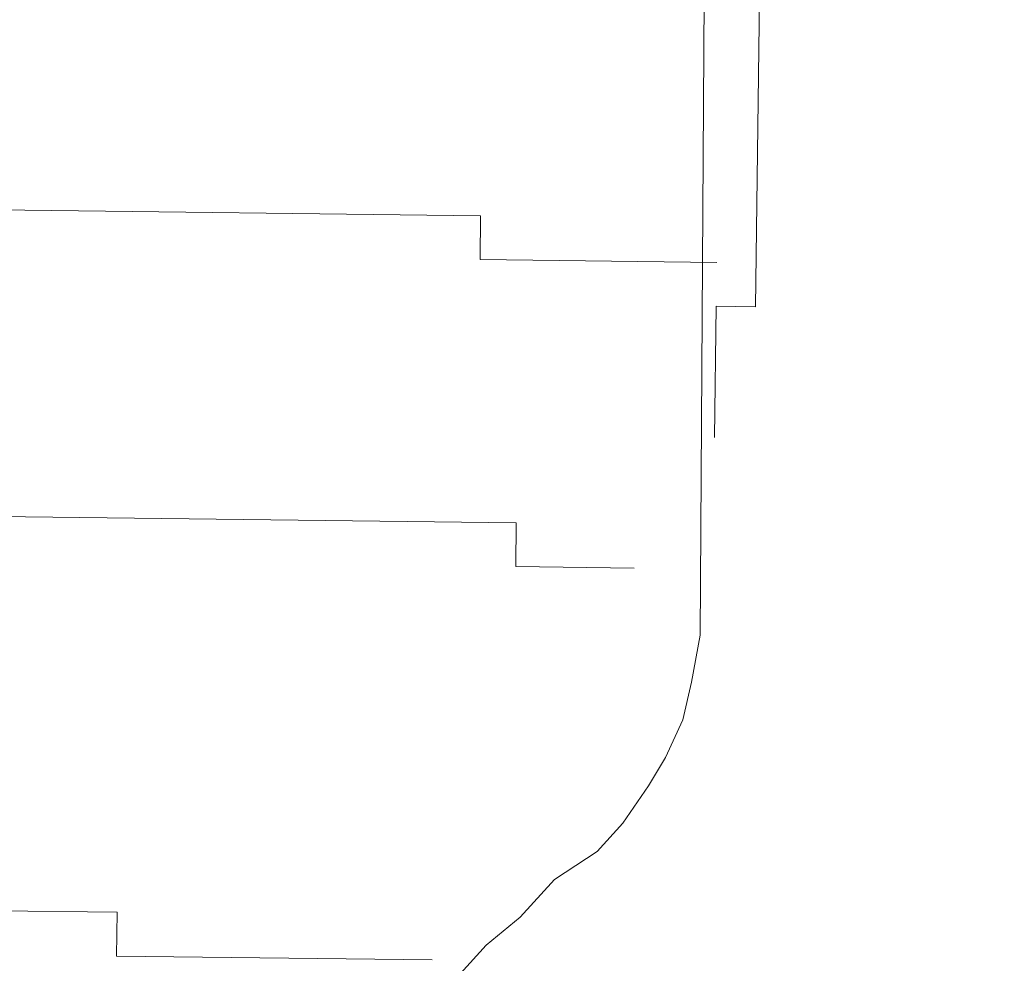
# Model space of a CAD drawing. Units: inches. Extents: x -466983 to 1020, y 324 to 318697.
# Tile 63 of 97: x 640.735 to 643.839, y 942.694 to 945.669. Entities that reach past the tile are written whole.
import ezdxf

# ---------------------------------------------------------------- set-up
doc = ezdxf.new("R2010")
doc.units = ezdxf.units.IN
doc.header["$MEASUREMENT"] = 0
doc.layers.add('A-FLOR-PATT', color=252, linetype='Continuous', lineweight=13)
doc.layers.add('A-FURN', color=8, linetype='Continuous', lineweight=18)

# ---------------------------------------------------------------- blocks, each defined once
blk = doc.blocks.new('L Shaped Sofa')
at = {"ltscale": 2}
for p, q in [((2421.6339, 743.6354), (2421.7812, 743.7974)), ((2421.9449, 743.7202), (2423.7596, 743.698)), ((2423.7596, 743.698), (2423.7566, 743.4461)), ((2421.4377, 743.4737), (2421.6339, 743.6354)), ((2421.2412, 743.2577), (2421.4377, 743.4737)), ((2423.7566, 743.4461), (2430.7885, 743.3602)), ((2420.9962, 743.0962), (2421.2412, 743.2577)), ((2420.8488, 742.9343), (2420.9962, 743.0962)), ((2420.7011, 742.7181), (2420.8488, 742.9343)), ((2420.6025, 742.5559), (2420.7011, 742.7181)), ((2420.5036, 742.3395), (2420.6025, 742.5559)), ((2420.4535, 742.1229), (2420.5036, 742.3395)), ((2420.403, 741.852), (2420.4535, 742.1229)), ((2420.3785, 737.84), (2420.403, 741.852)), ((2420.7831, 741.4668), (2421.4636, 741.4585)), ((2421.4636, 741.4585), (2421.4605, 741.2066)), ((2421.4605, 741.2066), (2432.3486, 741.0736)), ((2420.3109, 739.9609), (2420.3202, 740.7166)), ((2420.0564, 737.6965), (2420.0841, 739.9637)), ((2420.0841, 739.9637), (2420.3109, 739.9609)), ((2420.3078, 739.709), (2421.6689, 739.6924)), ((2421.6689, 739.6924), (2421.6658, 739.4404)), ((2421.6658, 739.4404), (2428.4709, 739.3573))]:
    blk.add_line(p, q, dxfattribs=at)

msp = doc.modelspace()

# ---------------------------------------------------------------- hatches: boundary and pattern name
at = {"layer": 'A-FLOR-PATT', "transparency": 33554572}
h = msp.add_hatch(dxfattribs=at)
h.set_pattern_fill('ANSI37', color=256, scale=30)
h.set_pattern_definition([(45, (-1212.4137, -290.035), (-2.6516504, 2.6516504), []), (135, (-1212.4137, -290.035), (-2.6516504, -2.6516504), [])])
h.paths.add_polyline_path([(901.8057, 1075.9377), (900.6144, 1075.9377), (900.6144, 1065.3856), (899.391, 1065.3856), (898.0911, 1065.3856), (892.8356, 1058.7098, -0.258377), (892.1875, 1058.3509), (879.9848, 1058.3509, -0.20177), (879.4382, 1058.5808), (874.0812, 1065.3856), (872.7813, 1065.3856), (871.5579, 1065.3856), (871.5579, 1075.9377), (813.8057, 1075.9377), (813.8057, 1044.7922), (832.3947, 1044.7922, -0.394795), (848.6602, 1028.5356), (848.6602, 1009.9377), (901.8057, 1009.9377), (901.8057, 1015.9377), (901.3057, 1015.9377), (871.3057, 1015.9377), (871.3057, 1017.2502), (871.3344, 1017.2502, -0.401453), (901.3057, 1045.9377), (901.8057, 1045.9377)])
edge = h.paths.add_edge_path(flags=16)
edge.add_line((847.7731, 1068.9486), (847.7731, 1073.7088))
edge.add_arc((849.2269, 1073.7088), 1.4538, 90, 180, ccw=False)
edge.add_line((849.2269, 1075.1627), (864.4921, 1075.1627))
edge.add_arc((864.4921, 1073.7088), 1.4538, 0, 90, ccw=False)
edge.add_line((865.9459, 1073.7088), (865.9459, 1069.0035))
edge.add_arc((832.6447, 1068.9761), 33.3012, -20.61234, 0.04725, ccw=False)
edge.add_ellipse((856.8595, 1058.48), major_axis=(0, 10.2131), ratio=0.6859192, start_angle=100.00884, end_angle=259.99116, ccw=False)
edge.add_arc((881.0742, 1068.9761), 33.3012, 180.04725, 200.61234, ccw=False)
h.paths.add_polyline_path([(853.1456, 1066.4815), (853.1456, 1066.4534), (853.1463, 1066.4534, 0.433107), (852.9166, 1066.6849), (852.9166, 1066.4534), (853.1456, 1066.4534), (853.1456, 1066.4815), (853.088, 1066.6122, 0.697939), (852.6995, 1066.4534), (852.7003, 1066.4534), (852.7003, 1066.4815), (852.9166, 1067.0012), (852.9166, 1066.6849, -0.396254)], flags=0)
h.paths.add_polyline_path([(861.0187, 1066.4815), (861.0187, 1066.4534), (861.0194, 1066.4534, 0.416404), (860.8024, 1066.6849), (860.8024, 1066.4534), (861.0187, 1066.4534), (861.0187, 1066.4815), (860.9672, 1066.6053, 0.713344), (860.5726, 1066.4534), (860.5734, 1066.4534), (860.5734, 1066.4815), (860.8024, 1067.0012), (860.8024, 1066.6849, -0.379973)], flags=0)
edge = h.paths.add_edge_path(flags=0)
edge.add_spline(control_points=[(861.1298, 1065.7855), (861.4661, 1065.2478), (861.6134, 1065.0161), (861.9833, 1064.3736), (862.1924, 1063.9443), (862.5614, 1063.0391), (862.7212, 1062.5633), (862.9865, 1061.5781), (863.092, 1061.0689), (863.2452, 1060.031), (863.293, 1059.5025), (863.3295, 1058.4409), (863.3181, 1057.9078), (863.2366, 1056.8518), (863.1664, 1056.3289), (862.9695, 1055.308), (862.8427, 1054.8099), (862.5365, 1053.8522), (862.3571, 1053.3927), (861.9514, 1052.5249), (861.7251, 1052.1166), (861.233, 1051.3622), (860.9672, 1051.0162), (860.4048, 1050.3949), (860.1082, 1050.1197), (859.4937, 1049.6461), (859.1758, 1049.4476), (858.5276, 1049.1299), (858.1973, 1049.0107), (857.5315, 1048.8518), (857.1959, 1048.8121), (856.5249, 1048.812), (856.1894, 1048.8515), (855.5236, 1049.0101), (855.1933, 1049.1291), (854.545, 1049.4465), (854.2271, 1049.6449), (853.6124, 1050.1183), (853.3158, 1050.3933), (852.7533, 1051.0143), (852.4874, 1051.3602), (851.9952, 1052.1144), (851.7688, 1052.5225), (851.3629, 1053.3902), (851.1834, 1053.8496), (850.877, 1054.8071), (850.7501, 1055.3051), (850.553, 1056.326), (850.4827, 1056.8488), (850.401, 1057.9048), (850.3895, 1058.4379), (850.4257, 1059.4995), (850.4734, 1060.0281), (850.6265, 1061.066), (850.7318, 1061.5753), (850.9969, 1062.5605), (851.1567, 1063.0365), (851.5254, 1063.9418), (851.7345, 1064.3712), (852.1056, 1065.0164), (852.2544, 1065.2503), (852.6082, 1065.7335)], knot_values=[3.915332, 3.915332, 3.915332, 3.915332, 4.013468, 4.013468, 4.175532, 4.175532, 4.337596, 4.337596, 4.49966, 4.49966, 4.661724, 4.661724, 4.823788, 4.823788, 4.985852, 4.985852, 5.147916, 5.147916, 5.30998, 5.30998, 5.472044, 5.472044, 5.634109, 5.634109, 5.796173, 5.796173, 5.958237, 5.958237, 6.120301, 6.120301, 6.282365, 6.282365, 6.444429, 6.444429, 6.606493, 6.606493, 6.768557, 6.768557, 6.930621, 6.930621, 7.092685, 7.092685, 7.254749, 7.254749, 7.416813, 7.416813, 7.578878, 7.578878, 7.740942, 7.740942, 7.903006, 7.903006, 8.06507, 8.06507, 8.227134, 8.227134, 8.389198, 8.389198, 8.551262, 8.551262, 8.65037, 8.65037, 8.65037, 8.65037], degree=3, periodic=0)
edge.add_line((852.6421, 1065.7855), (861.1298, 1065.7855))
edge = h.paths.add_edge_path(flags=0)
edge.add_ellipse((856.8496, 1057.7432), major_axis=(0, 7.7921), ratio=0.687861, start_angle=0, end_angle=360)
h.paths.add_polyline_path([(848.8634, 1069.3891), (848.8634, 1073.9605, -0.414214), (849.9538, 1075.0508), (863.7652, 1075.0508, -0.414214), (864.8555, 1073.9605), (864.8555, 1069.3891, -0.388936), (864.5237, 1069.027, -0.043561), (849.1953, 1069.027, -0.388936)], flags=0)
h.paths.add_polyline_path([(853.1006, 1068.1122, -1), (852.6775, 1068.1122, -1)], flags=0)
edge = h.paths.add_edge_path(flags=0)
edge.add_ellipse((856.8595, 1057.3378), major_axis=(0, 2.207), ratio=0.657164, start_angle=0, end_angle=360)
h.paths.add_polyline_path([(861.0415, 1068.1122, -1), (860.6184, 1068.1122, -1)], flags=0)
edge = h.paths.add_edge_path()
edge.add_line((573.9537, 1057.3412), (573.9537, 1075.9377))
edge.add_line((573.9537, 1075.9377), (558.7308, 1075.9377))
edge.add_line((558.7308, 1075.9377), (558.7308, 1065.3856))
edge.add_line((558.7308, 1065.3856), (557.5074, 1065.3856))
edge.add_line((557.5074, 1065.3856), (556.2075, 1065.3856))
edge.add_line((556.2075, 1065.3856), (550.952, 1058.7098))
edge.add_arc((550.3039, 1059.1155), 0.7646, 270, 327.9483, ccw=False)
edge.add_line((550.3039, 1058.3509), (538.1012, 1058.3509))
edge.add_arc((538.1012, 1059.1155), 0.7646, 224.3704, 270, ccw=False)
edge.add_line((537.5546, 1058.5808), (532.1976, 1065.3856))
edge.add_line((532.1976, 1065.3856), (530.8977, 1065.3856))
edge.add_line((530.8977, 1065.3856), (529.6743, 1065.3856))
edge.add_line((529.6743, 1065.3856), (529.6743, 1075.9377))
edge.add_line((529.6743, 1075.9377), (520.8057, 1075.9377))
edge.add_line((520.8057, 1075.9377), (520.8057, 1045.9377))
edge.add_line((520.8057, 1045.9377), (521.3057, 1045.9377))
edge.add_arc((521.3057, 1015.9377), 30, 2.50749, 90, ccw=False)
edge.add_line((551.277, 1017.2502), (551.3057, 1017.2502))
edge.add_line((551.3057, 1017.2502), (551.3057, 1015.9377))
edge.add_line((551.3057, 1015.9377), (520.8057, 1015.9377))
edge.add_line((520.8057, 1015.9377), (520.8057, 1009.9377))
edge.add_line((520.8057, 1009.9377), (559.1913, 1010.4022))
edge.add_arc((559.1913, 1011.856), 1.4538, 180, 270, ccw=False)
edge.add_line((557.7375, 1011.856), (557.7375, 1016.5613))
edge.add_arc((591.0386, 1016.5888), 33.3012, 159.38766, 180.04725, ccw=False)
edge.add_ellipse((566.8239, 1027.0848), major_axis=(0, 10.2131), ratio=0.6859192, start_angle=280.00884, end_angle=439.99116, ccw=False)
edge.add_arc((542.6091, 1016.5888), 33.3012, 0.04725, 20.61234, ccw=False)
edge.add_line((575.9103, 1016.6162), (575.9103, 1011.856))
edge.add_arc((574.4565, 1011.856), 1.4538, -90, 0, ccw=False)
edge.add_line((574.4565, 1010.4022), (608.8057, 1009.9377))
edge.add_line((608.8057, 1009.9377), (608.8057, 1041.0857))
edge.add_line((608.8057, 1041.0857), (590.2179, 1041.0857))
edge.add_arc((590.775, 1057.9074), 16.8309, 181.92775, 268.10321, ccw=False)
edge = h.paths.add_edge_path()
edge.add_ellipse((494.2443, 583.6204), major_axis=(0, 10.2131), ratio=0.6859192, start_angle=280.00884, end_angle=439.99116, ccw=False)
edge.add_arc((470.0296, 573.1243), 33.3012, 0.04725, 20.61234, ccw=False)
edge.add_line((503.3307, 573.1518), (503.3307, 568.3916))
edge.add_arc((501.8769, 568.3916), 1.4538, -90, 0, ccw=False)
edge.add_line((501.8769, 566.9377), (539.8057, 566.9377))
edge.add_line((539.8057, 566.9377), (539.8057, 572.9377))
edge.add_line((539.8057, 572.9377), (539.3057, 572.9377))
edge.add_line((539.3057, 572.9377), (509.3057, 572.9377))
edge.add_line((509.3057, 572.9377), (509.3057, 574.2502))
edge.add_line((509.3057, 574.2502), (509.3344, 574.2502))
edge.add_arc((539.3057, 572.9377), 30, 90, 177.49251, ccw=False)
edge.add_line((539.3057, 602.9377), (539.8057, 602.9377))
edge.add_line((539.8057, 602.9377), (539.8057, 626.9377))
edge.add_line((539.8057, 626.9377), (531.7718, 626.9377))
edge.add_line((531.7718, 626.9377), (531.7718, 616.3856))
edge.add_line((531.7718, 616.3856), (530.5484, 616.3856))
edge.add_line((530.5484, 616.3856), (529.2485, 616.3856))
edge.add_line((529.2485, 616.3856), (523.7105, 609.3509))
edge.add_line((523.7105, 609.3509), (510.7766, 609.3509))
edge.add_line((510.7766, 609.3509), (505.2386, 616.3856))
edge.add_line((505.2386, 616.3856), (503.9387, 616.3856))
edge.add_line((503.9387, 616.3856), (502.7153, 616.3856))
edge.add_line((502.7153, 616.3856), (502.7153, 626.9377))
edge.add_line((502.7153, 626.9377), (481.6983, 626.9377))
edge.add_line((481.6983, 626.9377), (481.6983, 610.995))
edge.add_arc((467.2703, 611.4728), 14.4359, 271.92775, 358.10321, ccw=False)
edge.add_line((467.7559, 597.0451), (451.8057, 597.0451))
edge.add_line((451.8057, 597.0451), (451.8057, 584.4035))
edge.add_line((451.8057, 584.4035), (451.8057, 566.9377))
edge.add_line((451.8057, 566.9377), (486.6117, 566.9377))
edge.add_arc((486.6117, 568.3916), 1.4538, 180, 270, ccw=False)
edge.add_line((485.1579, 568.3916), (485.1579, 573.0969))
edge.add_arc((518.4591, 573.1243), 33.3012, 159.38766, 180.04725, ccw=False)
h.paths.add_polyline_path([(836.2609, 1020.7328), (879.8898, 1020.7328), (879.8898, 1039.3902), (836.2609, 1039.3902)], flags=25)
h.paths.add_polyline_path([(549.9851, 1036.7492), (593.614, 1036.7492), (593.614, 1055.4065), (549.9851, 1055.4065)], flags=24)
h.paths.add_polyline_path([(475.123, 595.5959), (518.752, 595.5959), (518.752, 614.2532), (475.123, 614.2532)], flags=24)
h = msp.add_hatch(dxfattribs=at)
h.set_pattern_fill('ANSI37', color=256, scale=20)
h.set_pattern_definition([(45, (-1212.4137, -290.035), (-1.767767, 1.767767), []), (135, (-1212.4137, -290.035), (-1.767767, -1.767767), [])])
h.paths.add_polyline_path([(809.8057, 870.9377), (809.8057, 888.1519), (806.9985, 888.1519), (802.6624, 888.1519), (789.3832, 888.1519), (786.2846, 888.1519, -0.414214), (785.4991, 888.9374), (785.4991, 900.1959), (785.4991, 908.4696, -0.414214), (786.8082, 909.7787, -0.414214), (785.4991, 911.0878), (785.4991, 929.1015, -0.414214), (786.8082, 930.4106, -0.414214), (785.4991, 931.7197), (785.4991, 931.9039, -0.414214), (784.19, 930.5948), (766.7223, 930.5948, -0.412359), (765.4132, 931.8956, -0.413741), (764.1145, 930.5782), (744.5781, 930.422, -0.416556), (743.7864, 931.2075), (743.7864, 933.5153), (742.2154, 933.5153), (742.2154, 952.024, -0.001344), (743.7864, 952.1998), (743.7864, 953.9377), (678.5915, 953.9377), (678.5915, 951.1305), (678.5915, 946.7945), (678.5915, 933.5153), (678.5915, 930.4166, -0.414214), (677.806, 929.6312), (666.5475, 929.6312), (658.2738, 929.6312, -0.414214), (656.9647, 930.9403, -0.414214), (655.6556, 929.6312), (637.6419, 929.6312, -0.414214), (636.3328, 930.9403, -0.414214), (635.0237, 929.6312), (634.8395, 929.6312, -0.414214), (636.1486, 928.322), (636.1486, 910.8544, -0.412359), (634.8478, 909.5452, -0.413741), (636.1653, 908.2466), (636.3214, 888.7102, -0.416556), (635.5359, 887.9184), (633.2281, 887.9184), (633.2281, 886.3475), (614.7194, 886.3475, -0.001344), (614.5436, 887.9184), (612.8057, 887.9184), (612.8057, 834.9377), (612.8057, 752.9377), (612.8057, 748.9377), (612.8057, 697.9377), (654.8057, 697.9377), (654.8057, 701.9377), (715.8057, 701.9377), (715.8057, 737.4353), (774.2918, 737.4353), (774.2918, 795.9377), (809.8057, 795.9377)])
h.paths.add_polyline_path([(679.2761, 849.5757, 0.102523), (682.1475, 849.2608, -0.080461), (694.5428, 849.7725, -0.283899), (694.4822, 849.0082, 0.136605), (694.4068, 848.8103, -0.030441), (694.5428, 846.8929), (694.5428, 842.6198), (694.5428, 838.3466, -0.028219), (694.4246, 836.5684), (694.425, 836.5684, 0.196187), (694.4456, 836.2708, -0.302897), (694.5428, 835.467, -0.080461), (682.1475, 835.9787, 0.102523), (679.2761, 835.6638, -0.58611), (678.6457, 836.0169), (678.6457, 849.2227, -0.58611)], flags=16)
h.paths.add_polyline_path([(679.5173, 848.6515, 0.699597), (679.476, 848.6342, 1.20716), (679.1935, 848.7422, 0.010621)], flags=0)
h.paths.add_polyline_path([(679.4923, 836.5608, -0.013798), (679.9178, 836.6594, -0.071703), (682.8533, 837.1434, -0.165743), (682.1665, 839.1006), (682.1665, 842.6094), (682.1665, 846.0603, -0.240616), (683.4733, 848.6767, -0.068263), (693.9295, 849.0082), (693.7875, 848.7083), (693.7875, 849.0228, 0.067332), (683.4733, 848.6767, 0.240616), (682.1665, 846.0603), (682.1665, 842.6094), (682.1665, 839.1006, 0.23459), (683.461, 836.5513, 0.068093), (693.7875, 836.1955), (693.7875, 836.5104), (693.9296, 836.2102, -0.077215), (682.2421, 836.7815, 0.086627), (679.5283, 836.5701, -0.628402), (679.5029, 836.5735), (679.5029, 836.6071, 0.910458)], flags=0)
h.paths.add_polyline_path([(679.476, 848.6364), (679.2069, 848.647), (679.2069, 836.5718, 0.913566), (679.3645, 836.5861), (679.476, 836.5824)], flags=0)
h.paths.add_polyline_path([(679.2761, 829.8604, 0.102523), (682.1475, 829.5455, -0.080461), (694.5428, 830.0572, -0.283899), (694.4822, 829.2929, 0.136605), (694.4068, 829.095, -0.030441), (694.5428, 827.1776), (694.5428, 822.9045), (694.5428, 818.6314, -0.028219), (694.4246, 816.8531), (694.425, 816.8532, 0.196187), (694.4456, 816.5555, -0.302897), (694.5428, 815.7517, -0.080461), (682.1475, 816.2635, 0.102523), (679.2761, 815.9485, -0.58611), (678.6457, 816.3016), (678.6457, 829.5074, -0.58611)], flags=16)
h.paths.add_polyline_path([(679.5173, 828.9362, 0.699597), (679.476, 828.9189, 1.20716), (679.1935, 829.0269, 0.010621)], flags=0)
h.paths.add_polyline_path([(679.4923, 816.8456, -0.013798), (679.9178, 816.9441, -0.071703), (682.8533, 817.4281, -0.165743), (682.1665, 819.3853), (682.1665, 822.8941), (682.1665, 826.345, -0.240616), (683.4733, 828.9614, -0.068263), (693.9295, 829.2929), (693.7875, 828.9931), (693.7875, 829.3076, 0.067332), (683.4733, 828.9614, 0.240616), (682.1665, 826.345), (682.1665, 822.8941), (682.1665, 819.3853, 0.23459), (683.461, 816.836, 0.068093), (693.7875, 816.4802), (693.7875, 816.7952), (693.9296, 816.4949, -0.077215), (682.2421, 817.0662, 0.086627), (679.5283, 816.8549, -0.628402), (679.5029, 816.8582), (679.5029, 816.8918, 0.910458)], flags=0)
h.paths.add_polyline_path([(679.476, 828.9211), (679.2069, 828.9317), (679.2069, 816.8565, 0.913566), (679.3645, 816.8708), (679.476, 816.8671)], flags=0)
h.paths.add_polyline_path([(679.2761, 810.1451, 0.102523), (682.1475, 809.8302, -0.080461), (694.5428, 810.342, -0.3023), (694.4466, 809.5394, 0.10023), (694.4058, 809.3878, -0.03057), (694.5428, 807.4623), (694.5428, 803.1892), (694.5428, 798.9161, -0.03057), (694.4058, 796.9906, 0.10023), (694.4466, 796.839, -0.3023), (694.5428, 796.0365, -0.080461), (682.1475, 796.5482, 0.102523), (679.2761, 796.2333, -0.58611), (678.6457, 796.5863), (678.6457, 809.7921, -0.58611)], flags=16)
h.paths.add_polyline_path([(679.5173, 809.2417, 0.699597), (679.476, 809.2244, 1.20716), (679.1935, 809.3324, 0.010621)], flags=0)
h.paths.add_polyline_path([(679.4923, 797.151, -0.013798), (679.9178, 797.2496, -0.071703), (682.8533, 797.7336, -0.165743), (682.1665, 799.6908), (682.1665, 803.1996), (682.1665, 806.6505, -0.239349), (683.461, 809.2577, -0.072465), (694.4468, 809.5405, 0.197932), (694.425, 809.2405), (693.7875, 809.2985), (693.7875, 809.6135, 0.068093), (683.461, 809.2577, 0.239349), (682.1665, 806.6505), (682.1665, 803.1996), (682.1665, 799.6908, 0.235854), (683.4733, 797.1323, 0.067332), (693.7875, 796.7861), (693.7875, 797.1006), (694.425, 797.1586, 0.197932), (694.4468, 796.8586, -0.080419), (682.1557, 797.3795, 0.083867), (679.5283, 797.1603, -0.628402), (679.5029, 797.1637), (679.5029, 797.1973, 0.910458)], flags=0)
h.paths.add_polyline_path([(679.2069, 809.2372), (679.2069, 797.162, 0.913566), (679.3645, 797.1763), (679.476, 797.1726), (679.476, 809.2266)], flags=0)
h.paths.add_polyline_path([(695.3643, 853.2989), (728.2231, 853.2989), (728.2231, 771.1519), (695.3643, 771.1519)], flags=16)
h.paths.add_polyline_path([(696.0215, 852.6417), (727.5659, 852.6417), (727.5659, 771.809), (696.0215, 771.809)], flags=0)
h.paths.add_polyline_path([(679.2761, 788.7869, 0.102523), (682.1475, 788.472, -0.080461), (694.5428, 788.9837, -0.3023), (694.4466, 788.1812, 0.10023), (694.4058, 788.0296, -0.03057), (694.5428, 786.1041), (694.5428, 781.831), (694.5428, 777.5578, -0.03057), (694.4058, 775.6323, 0.10023), (694.4466, 775.4808, -0.3023), (694.5428, 774.6782, -0.080461), (682.1475, 775.19, 0.102523), (679.2761, 774.875, -0.58611), (678.6457, 775.2281), (678.6457, 788.4339, -0.58611)], flags=16)
h.paths.add_polyline_path([(679.5173, 787.8834, 0.699597), (679.476, 787.8662, 1.20716), (679.1935, 787.9742, 0.010621)], flags=0)
h.paths.add_polyline_path([(679.4923, 775.7928, -0.013798), (679.9178, 775.8914, -0.071703), (682.8533, 776.3753, -0.165743), (682.1665, 778.3325), (682.1665, 781.8414), (682.1665, 785.2922, -0.239349), (683.461, 787.8995, -0.072465), (694.4468, 788.1823, 0.197932), (694.425, 787.8823), (693.7875, 787.9403), (693.7875, 788.2553, 0.068093), (683.461, 787.8995, 0.239349), (682.1665, 785.2922), (682.1665, 781.8414), (682.1665, 778.3325, 0.235854), (683.4733, 775.7741, 0.067332), (693.7875, 775.4279), (693.7875, 775.7424), (694.425, 775.8004, 0.197932), (694.4468, 775.5004, -0.080419), (682.1557, 776.0212, 0.083867), (679.5283, 775.8021, -0.628402), (679.5029, 775.8054), (679.5029, 775.8391, 0.910458)], flags=0)
h.paths.add_polyline_path([(679.2069, 787.8789), (679.2069, 775.8038, 0.913566), (679.3645, 775.818), (679.476, 775.8144), (679.476, 787.8684)], flags=0)
h.paths.add_polyline_path([(704.641, 854.1204, -0.080461), (705.1527, 866.5157, 0.102523), (704.8378, 869.3871, -0.58611), (705.1908, 870.0174), (718.3966, 870.0174, -0.58611), (718.7496, 869.3871, 0.102523), (718.4347, 866.5157, -0.080461), (718.9465, 854.1204, -0.3023), (718.1439, 854.2166, 0.10023), (717.9924, 854.2574, -0.03057), (716.0668, 854.1204), (711.7937, 854.1204), (707.5206, 854.1204, -0.03057), (705.5951, 854.2574, 0.10023), (705.4435, 854.2166, -0.3023)], flags=16)
h.paths.add_polyline_path([(717.8462, 869.1459, 0.699597), (717.8289, 869.1872, 1.20716), (717.9369, 869.4697, 0.010621)], flags=0)
h.paths.add_polyline_path([(705.4631, 854.2164, -0.080419), (705.984, 866.5074, 0.083867), (705.7648, 869.1349, -0.628402), (705.7682, 869.1603), (705.8018, 869.1603, 0.910458), (705.7555, 869.1709, -0.013798), (705.8541, 868.7454, -0.071703), (706.3381, 865.8099, -0.165743), (708.2953, 866.4967), (711.8041, 866.4967), (715.255, 866.4967, -0.239349), (717.8622, 865.2022, -0.072465), (718.145, 854.2164, 0.197932), (717.845, 854.2382), (717.903, 854.8757), (718.218, 854.8757, 0.068093), (717.8622, 865.2022, 0.239349), (715.255, 866.4967), (711.8041, 866.4967), (708.2953, 866.4967, 0.235854), (705.7368, 865.1898, 0.067332), (705.3906, 854.8757), (705.7051, 854.8757), (705.7631, 854.2382, 0.197932)], flags=16)
h.paths.add_polyline_path([(705.7665, 869.4563, 0.913566), (705.7808, 869.2987), (705.7771, 869.1872), (717.8311, 869.1872), (717.8417, 869.4563)], flags=0)
h.paths.add_polyline_path([(729.0446, 842.6198), (729.0446, 846.8929, -0.03057), (729.1817, 848.8184, 0.10023), (729.1408, 848.9699, -0.3023), (729.0446, 849.7725, -0.080461), (741.4399, 849.2608, 0.102523), (744.3113, 849.5757, -0.58611), (744.9417, 849.2227), (744.9417, 836.0169, -0.58611), (744.3113, 835.6638, 0.102523), (741.4399, 835.9787, -0.080461), (729.0446, 835.467, -0.3023), (729.1408, 836.2696, 0.10023), (729.1817, 836.4211, -0.03057), (729.0446, 838.3466)], flags=16)
h.paths.add_polyline_path([(744.1115, 836.5846, 1.20716), (744.3939, 836.4766, 0.010621), (744.0701, 836.5673, 0.699597)], flags=0)
h.paths.add_polyline_path([(729.1407, 836.2684, 0.197932), (729.1624, 836.5684), (729.7999, 836.5104), (729.7999, 836.1955, 0.068093), (740.1264, 836.5513, 0.239349), (741.4209, 839.1585), (741.4209, 842.6094), (741.4209, 846.1182, 0.235854), (740.1141, 848.6767, 0.067332), (729.7999, 849.0228), (729.7999, 848.7083), (729.1624, 848.6503, 0.197932), (729.1407, 848.9504, -0.080419), (741.4317, 848.4295, 0.083867), (744.0591, 848.6486, -0.628402), (744.0845, 848.6453), (744.0845, 848.6117, 0.910458), (744.0951, 848.6579, -0.013798), (743.6696, 848.5594, -0.071703), (740.7341, 848.0754, -0.165743), (741.4209, 846.1182), (741.4209, 842.6094), (741.4209, 839.1585, -0.239349), (740.1264, 836.5513, -0.072465)], flags=0)
h.paths.add_polyline_path([(729.0446, 830.0572, -0.080461), (741.4399, 829.5455, 0.102523), (744.3113, 829.8604, -0.58611), (744.9417, 829.5074), (744.9417, 816.3016, -0.58611), (744.3113, 815.9485, 0.102523), (741.4399, 816.2635, -0.080461), (729.0446, 815.7517, -0.3023), (729.1408, 816.5543, 0.10023), (729.1817, 816.7058, -0.03057), (729.0446, 818.6314), (729.0446, 822.9045), (729.0446, 827.1776, -0.03057), (729.1817, 829.1031, 0.10023), (729.1408, 829.2547, -0.3023)], flags=16)
h.paths.add_polyline_path([(744.1115, 816.8693, 1.20716), (744.3939, 816.7613, 0.010621), (744.0701, 816.852, 0.699597)], flags=0)
h.paths.add_polyline_path([(729.1407, 829.2351, -0.080419), (741.4317, 828.7142, 0.083867), (744.0591, 828.9334, -0.628402), (744.0845, 828.93), (744.0845, 828.8964, 0.910458), (744.0951, 828.9427, -0.013798), (743.6696, 828.8441, -0.071703), (740.7341, 828.3601, -0.165743), (741.4209, 826.4029), (741.4209, 822.8941), (741.4209, 819.4432, -0.239349), (740.1264, 816.836, -0.072465), (729.1407, 816.5531, 0.197932), (729.1624, 816.8532), (729.7999, 816.7952), (729.7999, 816.4802, 0.068093), (740.1264, 816.836, 0.239349), (741.4209, 819.4432), (741.4209, 822.8941), (741.4209, 826.4029, 0.235854), (740.1141, 828.9614, 0.067332), (729.7999, 829.3076), (729.7999, 828.9931), (729.1624, 828.9351, 0.197932)], flags=16)
h.paths.add_polyline_path([(729.0446, 810.342, -0.080461), (741.4399, 809.8302, 0.102523), (744.3113, 810.1451, -0.58611), (744.9417, 809.7921), (744.9417, 796.5863, -0.58611), (744.3113, 796.2333, 0.102523), (741.4399, 796.5482, -0.080461), (729.0446, 796.0365, -0.283899), (729.1052, 796.8007, 0.136605), (729.1806, 796.9987, -0.030441), (729.0446, 798.9161), (729.0446, 803.1892), (729.0446, 807.4623, -0.028219), (729.1628, 809.2406), (729.1624, 809.2405, 0.196187), (729.1418, 809.5382, -0.302897)], flags=16)
h.paths.add_polyline_path([(744.1115, 797.1748, 1.20716), (744.3939, 797.0668, 0.010621), (744.0701, 797.1575, 0.699597)], flags=0)
h.paths.add_polyline_path([(741.3453, 809.0275, 0.086627), (744.0591, 809.2388, -0.628402), (744.0845, 809.2355), (744.0845, 809.2019, 0.910458), (744.0951, 809.2481, -0.013798), (743.6696, 809.1496, -0.071703), (740.7341, 808.6656, -0.165743), (741.4209, 806.7084), (741.4209, 803.1996), (741.4209, 799.7487, -0.240616), (740.1141, 797.1323, -0.068263), (729.658, 796.8008), (729.7999, 797.1006), (729.7999, 796.7861, 0.067332), (740.1141, 797.1323, 0.240616), (741.4209, 799.7487), (741.4209, 803.1996), (741.4209, 806.7084, 0.23459), (740.1264, 809.2577, 0.068093), (729.7999, 809.6135), (729.7999, 809.2985), (729.6578, 809.5988, -0.077215)], flags=0)
h.paths.add_polyline_path([(704.641, 770.3304, -0.283899), (705.4053, 770.2697, 0.136605), (705.6032, 770.1944, -0.030441), (707.5206, 770.3304), (711.7937, 770.3304), (716.0668, 770.3304, -0.028219), (717.8451, 770.2122), (717.845, 770.2126, 0.196187), (718.1427, 770.2331, -0.302897), (718.9465, 770.3304, -0.080461), (718.4347, 757.9351, 0.102523), (718.7496, 755.0637, -0.58611), (718.3966, 754.4333), (705.1908, 754.4333, -0.58611), (704.8378, 755.0637, 0.102523), (705.1527, 757.9351, -0.080461)], flags=16)
h.paths.add_polyline_path([(705.762, 755.3048, 0.699597), (705.7793, 755.2635, 1.20716), (705.6713, 754.9811, 0.010621)], flags=0)
h.paths.add_polyline_path([(705.4053, 769.717), (705.7051, 769.5751), (705.3906, 769.5751, 0.067332), (705.7368, 759.2609, 0.240616), (708.3532, 757.954), (711.8041, 757.954), (715.3129, 757.954, 0.23459), (717.8622, 759.2485, 0.068093), (718.218, 769.5751), (717.903, 769.5751), (718.2033, 769.7172, -0.077215), (717.632, 758.0297, 0.086627), (717.8433, 755.3159, -0.628402), (717.84, 755.2904), (717.8064, 755.2904, 0.910458), (717.8526, 755.2799, -0.013798), (717.7541, 755.7053, -0.071703), (717.2701, 758.6409, -0.165743), (715.3129, 757.954), (711.8041, 757.954), (708.3532, 757.954, -0.240616), (705.7368, 759.2609, -0.068263)], flags=0)
h.paths.add_polyline_path([(729.0446, 788.9837, -0.080461), (741.4399, 788.472, 0.102523), (744.3113, 788.7869, -0.58611), (744.9417, 788.4339), (744.9417, 775.2281, -0.58611), (744.3113, 774.875, 0.102523), (741.4399, 775.19, -0.080461), (729.0446, 774.6782, -0.283899), (729.1052, 775.4425, 0.136605), (729.1806, 775.6405, -0.030441), (729.0446, 777.5578), (729.0446, 781.831), (729.0446, 786.1041, -0.028219), (729.1628, 787.8823), (729.1624, 787.8823, 0.196187), (729.1418, 788.1799, -0.302897)], flags=16)
h.paths.add_polyline_path([(744.1115, 775.8165, 1.20716), (744.3939, 775.7086, 0.010621), (744.0701, 775.7993, 0.699597)], flags=0)
h.paths.add_polyline_path([(741.3453, 787.6692, 0.086627), (744.0591, 787.8806, -0.628402), (744.0845, 787.8773), (744.0845, 787.8437, 0.910458), (744.0951, 787.8899, -0.013798), (743.6696, 787.7913, -0.071703), (740.7341, 787.3074, -0.165743), (741.4209, 785.3502), (741.4209, 781.8414), (741.4209, 778.3905, -0.240616), (740.1141, 775.7741, -0.068263), (729.658, 775.4425), (729.7999, 775.7424), (729.7999, 775.4279, 0.067332), (740.1141, 775.7741, 0.240616), (741.4209, 778.3905), (741.4209, 781.8414), (741.4209, 785.3502, 0.23459), (740.1264, 787.8995, 0.068093), (729.7999, 788.2553), (729.7999, 787.9403), (729.6578, 788.2405, -0.077215)], flags=0)
h.paths.add_polyline_path([(744.1115, 848.6364), (744.1115, 836.5824), (744.3805, 836.5718), (744.3805, 848.647, 0.913566), (744.2229, 848.6327)], flags=0)
h.paths.add_polyline_path([(744.2229, 828.9174), (744.1115, 828.9211), (744.1115, 816.8671), (744.3805, 816.8565), (744.3805, 828.9317, 0.913566)], flags=0)
h.paths.add_polyline_path([(717.8311, 755.2635), (705.7771, 755.2635), (705.7665, 754.9945), (717.8417, 754.9945, 0.913566), (717.8274, 755.1521)], flags=0)
h.paths.add_polyline_path([(744.2229, 809.2229), (744.1115, 809.2266), (744.1115, 797.1726), (744.3805, 797.162), (744.3805, 809.2372, 0.913566)], flags=0)
h.paths.add_polyline_path([(744.1115, 787.8684), (744.1115, 775.8144), (744.3805, 775.8038), (744.3805, 787.8789, 0.913566), (744.2229, 787.8647)], flags=0)
h.paths.add_polyline_path([(678.8774, 877.1228), (737.6127, 877.1228), (737.6127, 899.5116), (678.8774, 899.5116)], flags=24)

# ---------------------------------------------------------------- linework, layer by layer
at = {"layer": 'A-FURN', "ltscale": 2}
for p, q in [((643.0707, 946.0067), (643.0555, 944.7638)), ((643.0707, 946.0067), (643.0555, 944.7638)), ((643.0707, 946.0067), (643.0555, 944.7638)), ((643.0707, 946.0067), (643.0555, 944.7638)), ((643.0707, 946.0067), (643.0555, 944.7638)), ((643.0707, 946.0067), (643.0555, 944.7638)), ((642.8941, 945.928), (642.8807, 943.7285)), ((642.8941, 945.928), (642.8807, 943.7285)), ((642.8941, 945.928), (642.8807, 943.7285)), ((642.8941, 945.928), (642.8807, 943.7285)), ((642.8941, 945.928), (642.8807, 943.7285)), ((642.8941, 945.928), (642.8807, 943.7285)), ((642.1884, 945.0506), (638.4577, 945.0962)), ((642.1884, 945.0506), (638.4577, 945.0962)), ((642.1884, 945.0506), (638.4577, 945.0962)), ((642.1884, 945.0506), (638.4577, 945.0962)), ((642.1884, 945.0506), (638.4577, 945.0962)), ((642.1884, 945.0506), (638.4577, 945.0962)), ((642.1867, 944.9125), (642.1884, 945.0506)), ((642.1867, 944.9125), (642.1884, 945.0506)), ((642.1867, 944.9125), (642.1884, 945.0506)), ((642.1867, 944.9125), (642.1884, 945.0506)), ((642.1867, 944.9125), (642.1884, 945.0506)), ((642.1867, 944.9125), (642.1884, 945.0506)), ((642.9328, 944.9034), (642.1867, 944.9125)), ((642.9328, 944.9034), (642.1867, 944.9125)), ((642.9328, 944.9034), (642.1867, 944.9125)), ((642.9328, 944.9034), (642.1867, 944.9125)), ((642.9328, 944.9034), (642.1867, 944.9125)), ((642.9328, 944.9034), (642.1867, 944.9125)), ((642.9311, 944.7653), (642.9261, 944.351)), ((642.9311, 944.7653), (642.9261, 944.351)), ((642.9311, 944.7653), (642.9261, 944.351)), ((642.9311, 944.7653), (642.9261, 944.351)), ((642.9311, 944.7653), (642.9261, 944.351)), ((642.9311, 944.7653), (642.9261, 944.351)), ((643.0555, 944.7638), (642.9311, 944.7653)), ((643.0555, 944.7638), (642.9311, 944.7653)), ((643.0555, 944.7638), (642.9311, 944.7653)), ((643.0555, 944.7638), (642.9311, 944.7653)), ((643.0555, 944.7638), (642.9311, 944.7653)), ((643.0555, 944.7638), (642.9311, 944.7653)), ((642.3009, 944.0824), (636.3319, 944.1553)), ((642.3009, 944.0824), (636.3319, 944.1553)), ((642.3009, 944.0824), (636.3319, 944.1553)), ((642.3009, 944.0824), (636.3319, 944.1553)), ((642.3009, 944.0824), (636.3319, 944.1553)), ((642.3009, 944.0824), (636.3319, 944.1553)), ((642.2992, 943.9443), (642.3009, 944.0824)), ((642.2992, 943.9443), (642.3009, 944.0824)), ((642.2992, 943.9443), (642.3009, 944.0824)), ((642.2992, 943.9443), (642.3009, 944.0824)), ((642.2992, 943.9443), (642.3009, 944.0824)), ((642.2992, 943.9443), (642.3009, 944.0824)), ((642.6723, 943.9397), (642.2992, 943.9443)), ((642.6723, 943.9397), (642.2992, 943.9443)), ((642.6723, 943.9397), (642.2992, 943.9443)), ((642.6723, 943.9397), (642.2992, 943.9443)), ((642.6723, 943.9397), (642.2992, 943.9443)), ((642.6723, 943.9397), (642.2992, 943.9443)), ((642.8807, 943.7285), (642.853, 943.5801)), ((642.8807, 943.7285), (642.853, 943.5801)), ((642.8807, 943.7285), (642.853, 943.5801)), ((642.8807, 943.7285), (642.853, 943.5801)), ((642.8807, 943.7285), (642.853, 943.5801)), ((642.8807, 943.7285), (642.853, 943.5801)), ((642.853, 943.5801), (642.8255, 943.4613)), ((642.853, 943.5801), (642.8255, 943.4613)), ((642.853, 943.5801), (642.8255, 943.4613)), ((642.853, 943.5801), (642.8255, 943.4613)), ((642.853, 943.5801), (642.8255, 943.4613)), ((642.853, 943.5801), (642.8255, 943.4613)), ((642.8255, 943.4613), (642.7713, 943.3427)), ((642.8255, 943.4613), (642.7713, 943.3427)), ((642.8255, 943.4613), (642.7713, 943.3427)), ((642.8255, 943.4613), (642.7713, 943.3427)), ((642.8255, 943.4613), (642.7713, 943.3427)), ((642.8255, 943.4613), (642.7713, 943.3427)), ((642.7713, 943.3427), (642.7172, 943.2537)), ((642.7713, 943.3427), (642.7172, 943.2537)), ((642.7713, 943.3427), (642.7172, 943.2537)), ((642.7713, 943.3427), (642.7172, 943.2537)), ((642.7713, 943.3427), (642.7172, 943.2537)), ((642.7713, 943.3427), (642.7172, 943.2537)), ((642.7172, 943.2537), (642.6363, 943.1352)), ((642.7172, 943.2537), (642.6363, 943.1352)), ((642.7172, 943.2537), (642.6363, 943.1352)), ((642.7172, 943.2537), (642.6363, 943.1352)), ((642.7172, 943.2537), (642.6363, 943.1352)), ((642.7172, 943.2537), (642.6363, 943.1352)), ((642.6363, 943.1352), (642.5555, 943.0464)), ((642.6363, 943.1352), (642.5555, 943.0464)), ((642.6363, 943.1352), (642.5555, 943.0464)), ((642.6363, 943.1352), (642.5555, 943.0464)), ((642.6363, 943.1352), (642.5555, 943.0464)), ((642.6363, 943.1352), (642.5555, 943.0464)), ((642.5555, 943.0464), (642.4212, 942.9579)), ((642.5555, 943.0464), (642.4212, 942.9579)), ((642.5555, 943.0464), (642.4212, 942.9579)), ((642.5555, 943.0464), (642.4212, 942.9579)), ((642.5555, 943.0464), (642.4212, 942.9579)), ((642.5555, 943.0464), (642.4212, 942.9579)), ((642.4212, 942.9579), (642.3134, 942.8395)), ((642.4212, 942.9579), (642.3134, 942.8395)), ((642.4212, 942.9579), (642.3134, 942.8395)), ((642.4212, 942.9579), (642.3134, 942.8395)), ((642.4212, 942.9579), (642.3134, 942.8395)), ((642.4212, 942.9579), (642.3134, 942.8395)), ((641.0422, 942.8546), (637.1872, 942.9017)), ((641.0422, 942.8546), (637.1872, 942.9017)), ((641.0422, 942.8546), (637.1872, 942.9017)), ((641.0422, 942.8546), (637.1872, 942.9017)), ((641.0422, 942.8546), (637.1872, 942.9017)), ((641.0422, 942.8546), (637.1872, 942.9017)), ((641.0405, 942.7165), (641.0422, 942.8546)), ((641.0405, 942.7165), (641.0422, 942.8546)), ((641.0405, 942.7165), (641.0422, 942.8546)), ((641.0405, 942.7165), (641.0422, 942.8546)), ((641.0405, 942.7165), (641.0422, 942.8546)), ((641.0405, 942.7165), (641.0422, 942.8546)), ((642.3134, 942.8395), (642.2059, 942.7509)), ((642.3134, 942.8395), (642.2059, 942.7509)), ((642.3134, 942.8395), (642.2059, 942.7509)), ((642.3134, 942.8395), (642.2059, 942.7509)), ((642.3134, 942.8395), (642.2059, 942.7509)), ((642.3134, 942.8395), (642.2059, 942.7509)), ((642.2059, 942.7509), (642.1251, 942.6621)), ((642.2059, 942.7509), (642.1251, 942.6621)), ((642.2059, 942.7509), (642.1251, 942.6621)), ((642.2059, 942.7509), (642.1251, 942.6621)), ((642.2059, 942.7509), (642.1251, 942.6621)), ((642.2059, 942.7509), (642.1251, 942.6621)), ((642.0353, 942.7044), (641.0405, 942.7165)), ((642.0353, 942.7044), (641.0405, 942.7165)), ((642.0353, 942.7044), (641.0405, 942.7165)), ((642.0353, 942.7044), (641.0405, 942.7165)), ((642.0353, 942.7044), (641.0405, 942.7165)), ((642.0353, 942.7044), (641.0405, 942.7165))]:
    msp.add_line(p, q, dxfattribs=at)

# ---------------------------------------------------------------- block references
at = {"layer": 'A-FURN', "xscale": 0.5482153745360612, "yscale": 0.5482153745360612, "zscale": 0.5482153745360612, "rotation": 180}
msp.add_blockref('L Shaped Sofa', (1969.7828, 1350.4232), dxfattribs=at)

doc.saveas('drawing.dxf')
